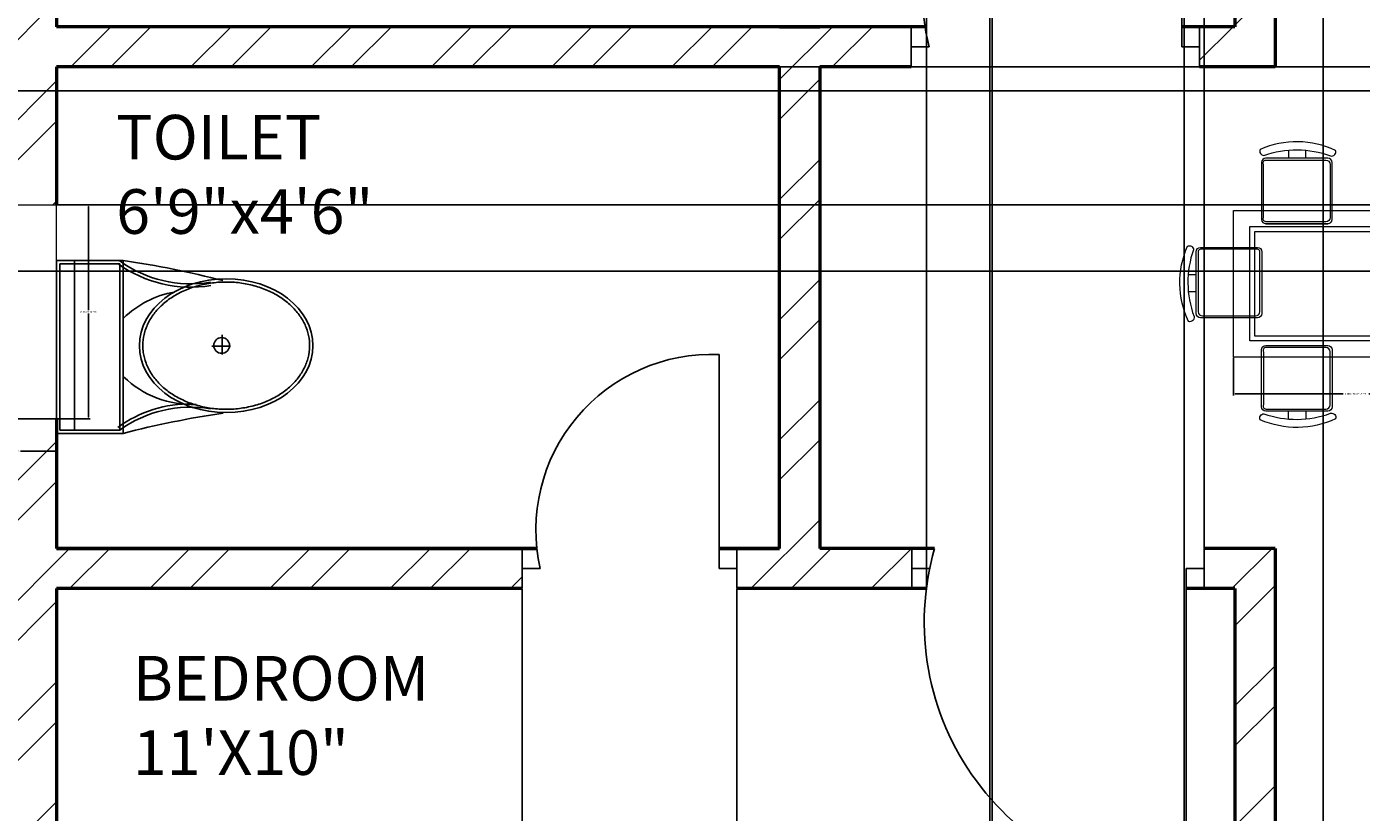
# Model space of a CAD drawing. Units: inches. Extents: x 1980 to 2738, y 1471 to 2568.
# Tile 4 of 22: x 2111 to 2260, y 1790 to 1878. Entities that reach past the tile are written whole.
import ezdxf

# ---------------------------------------------------------------- set-up
doc = ezdxf.new("R2010")
doc.units = ezdxf.units.IN
for name, color, linetype, lineweight in [('A-ANNO-DIMS', 2, 'Continuous', 18), ('A-AREA-IDEN', 7, 'Continuous', 18), ('A-DOOR', 31, 'Continuous', 25), ('A-FLOR-FIXT', 8, 'Continuous', 25), ('A-FURN', 8, 'Continuous', 18), ('A-GLAZ', 141, 'Continuous', 18), ('A-WALL', 7, 'Continuous', 50)]:
    doc.layers.add(name, color=color, linetype=linetype, lineweight=lineweight)
doc.layers.add('A-WALL-PATT', color=9, linetype='Continuous', lineweight=13, true_color=0xd19cc7)
doc.styles.get("Standard").update_dxf_attribs({"font": 'arial.ttf'})
doc.dimstyles.get("Standard").update_dxf_attribs({"dimtxt": 0.18, "dimasz": 0.18, "dimexe": 0.18, "dimexo": 0.0625, "dimgap": 0.09, "dimtad": 0, "dimtih": 1, "dimtoh": 1, "dimdec": 4, "dimzin": 0, "dimdsep": 46, "dimtxsty": 'Standard', "dimcen": 0.09, "dimadec": 0, "dimazin": 0, "dimtfac": 1, "dimtdec": 4, "dimtofl": 0, "dimtmove": 0, "dimatfit": 3, "dimfxl": 1, "dimtolj": 1, "dimtzin": 0, "dimarcsym": 0})

# ---------------------------------------------------------------- blocks, each defined once
blk = doc.blocks.new('A$C31115884')
for p, q in [((257.5, 466.4), (257.5, 523.2)), ((283.1, 497.7), (223.4, 497.7)), ((0, 200), (0, 0)), ((520, 200), (0, 200)), ((10, 190), (10, 10)), ((510, 190), (10, 190)), ((510, 10), (510, 190)), ((520, 0), (520, 200)), ((510, 54.5), (0, 54.5)), ((10, 10), (510, 10)), ((0, 0), (520, 0))]:
    blk.add_line(p, q)
blk.add_circle((255.6, 496.4), 23.6)
for centre, radius, start, end in [((2777.7, -204.6), 2807, 165.4549, 171.7133), ((3237, 905), 2807, 188.2867, 194.5451), ((-294.5, 403.3), 364.7, 324.2091, 9.3499), ((-294.5, 403.3), 374.7, 324.2091, 9.3499), ((805.8, 403.3), 364.7, 170.6501, 215.7909), ((139.5, 406.2), 293.5, 315.8436, 2.6563), ((805.8, 403.3), 374.7, 179.2036, 215.7909), ((383.6, 406.2), 293.5, 190.2774, 224.1564)]:
    blk.add_arc(centre, radius, start, end)
blk.add_ellipse((256.2, 509.9), major_axis=(0, -260.7), ratio=0.772727)
blk.add_open_spline([(256.2, 259.2), (263.1, 259.2), (270, 259.7), (287.8, 262.3), (298.7, 265.1), (319.9, 273.1), (330.2, 278.4), (350.1, 291.1), (359.7, 298.7), (377.7, 315.9), (386.2, 325.5), (401.7, 346.6), (408.8, 358.1), (421.3, 382.5), (426.8, 395.5), (435.9, 422.4), (439.5, 436.4), (444.8, 465.1), (446.5, 479.7), (447.9, 509.2), (447.6, 524), (445, 553.3), (442.7, 567.8), (436.3, 596), (432.1, 609.7), (421.9, 636), (416, 648.6), (402.5, 672.1), (395, 683), (378.6, 703), (369.8, 712.1), (351.1, 728), (341.3, 734.8), (320.9, 746.2), (310.4, 750.7), (288.9, 757.3), (278, 759.4), (256, 761), (245, 760.6), (223.1, 757.2), (212.3, 754.3), (191.1, 746.1), (180.8, 740.7), (160.9, 727.8), (151.4, 720.1), (133.5, 702.7), (125.1, 693), (109.6, 671.7), (102.6, 660.2), (90.2, 635.7), (84.9, 622.7), (76, 595.6), (72.4, 581.6), (67.2, 552.9), (65.6, 538.2), (64.4, 508.8), (64.8, 494), (67.5, 464.7), (69.9, 450.2), (76.6, 422), (80.8, 408.3), (91.1, 382.2), (97.2, 369.7), (110.8, 346.3), (118.4, 335.4), (134.8, 315.6), (143.7, 306.7), (162.4, 290.9), (172.3, 284.2), (192.8, 273), (203.3, 268.6), (224.8, 262.2), (235.8, 260.2), (249.9, 259.3), (253, 259.2), (256.2, 259.2)], degree=3, knots=[0, 0, 0, 0, 0.110105, 0.110105, 0.285049, 0.285049, 0.459994, 0.459994, 0.634938, 0.634938, 0.809882, 0.809882, 0.984827, 0.984827, 1.159771, 1.159771, 1.334715, 1.334715, 1.50966, 1.50966, 1.684604, 1.684604, 1.859549, 1.859549, 2.034493, 2.034493, 2.209437, 2.209437, 2.384382, 2.384382, 2.559326, 2.559326, 2.73427, 2.73427, 2.909215, 2.909215, 3.084159, 3.084159, 3.259103, 3.259103, 3.434048, 3.434048, 3.608992, 3.608992, 3.783936, 3.783936, 3.958881, 3.958881, 4.133825, 4.133825, 4.30877, 4.30877, 4.483714, 4.483714, 4.658658, 4.658658, 4.833603, 4.833603, 5.008547, 5.008547, 5.183491, 5.183491, 5.358436, 5.358436, 5.53338, 5.53338, 5.708324, 5.708324, 5.883269, 5.883269, 6.058213, 6.058213, 6.233158, 6.233158, 6.283185, 6.283185, 6.283185, 6.283185])
blk = doc.blocks.new('TABLE-DINING-RECT')
for points in [[(0, 16.47), (27.45, 16.47), (27.45, 0), (0, 0)], [(0, 16.47), (27.45, 16.47), (27.45, 0), (0, 0)], [(1.83, 14.64), (25.62, 14.64), (25.62, 1.83), (1.83, 1.83)], [(1.83, 14.64), (25.62, 14.64), (25.62, 1.83), (1.83, 1.83)], [(2.38, 14.09), (25.07, 14.09), (25.07, 2.38), (2.38, 2.38)], [(2.38, 14.09), (25.07, 14.09), (25.07, 2.38), (2.38, 2.38)]]:
    blk.add_lwpolyline(points, close=True)
blk = doc.blocks.new('WIN-24IN-WALL')
for p, q in [((4.5, 24), (0, 24)), ((0, 24), (9, 24)), ((0, 24), (0, 0)), ((4.5, 0), (4.5, 24)), ((9, 0), (9, 24)), ((0, 0), (9, 0)), ((9, 0), (4.5, 0))]:
    blk.add_line(p, q)
blk = doc.blocks.new('*D21')
at = {"layer": 'A-ANNO-DIMS', "color": 0, "lineweight": -2, "transparency": 16777216}
for p, q in [((2245.93, 1840.58), (2245.93, 1836.35)), ((2273.38, 1840.58), (2273.38, 1836.35)), ((2246.11, 1836.53), (2258.22, 1836.53)), ((2273.2, 1836.53), (2261.09, 1836.53))]:
    blk.add_line(p, q, dxfattribs=at)
at = {"layer": 'A-ANNO-DIMS', "color": 0, "transparency": 16777216}
for points in [[(2246.11, 1836.56), (2246.11, 1836.5), (2245.93, 1836.53)], [(2273.2, 1836.56), (2273.2, 1836.5), (2273.38, 1836.53)]]:
    blk.add_solid(points, dxfattribs=at)
at = {"layer": 'Defpoints', "color": 0, "transparency": 16777216}
for p in [(2245.93, 1840.64), (2273.38, 1840.64), (2273.38, 1836.53)]:
    blk.add_point(p, dxfattribs=at)
at = {"layer": 'A-ANNO-DIMS', "color": 0, "transparency": 16777216, "insert": (2259.65, 1836.53), "char_height": 0.18, "attachment_point": 5}
blk.add_mtext('\\A1;DINING TABLE 27 TYP.', dxfattribs=at)
blk = doc.blocks.new('*D23')
at = {"layer": 'A-ANNO-DIMS', "color": 0, "lineweight": -2, "transparency": 16777216}
for p, q in [((2114.15, 1857.73), (2117.86, 1857.73)), ((2117.68, 1857.55), (2117.68, 1845.91)), ((2117.68, 1833.91), (2117.68, 1845.54)), ((2114.15, 1833.73), (2117.86, 1833.73))]:
    blk.add_line(p, q, dxfattribs=at)
at = {"layer": 'A-ANNO-DIMS', "color": 0, "transparency": 16777216}
for points in [[(2117.65, 1857.55), (2117.71, 1857.55), (2117.68, 1857.73)], [(2117.65, 1833.91), (2117.71, 1833.91), (2117.68, 1833.73)]]:
    blk.add_solid(points, dxfattribs=at)
at = {"layer": 'Defpoints', "color": 0, "transparency": 16777216}
for p in [(2114.08, 1857.73), (2117.68, 1857.73), (2114.08, 1833.73)]:
    blk.add_point(p, dxfattribs=at)
at = {"layer": 'A-ANNO-DIMS', "color": 0, "transparency": 16777216, "insert": (2117.68, 1845.73), "char_height": 0.18, "attachment_point": 5}
blk.add_mtext('\\A1;WINDOW 24 TYP.', dxfattribs=at)
blk = doc.blocks.new('*D24')
at = {"layer": 'A-ANNO-DIMS', "color": 0, "lineweight": -2, "transparency": 16777216}
for p, q in [((2105.08, 1833.67), (2105.08, 1829.95)), ((2114.08, 1833.67), (2114.08, 1829.95)), ((2105.26, 1830.13), (2109.13, 1830.13)), ((2113.9, 1830.13), (2110.04, 1830.13))]:
    blk.add_line(p, q, dxfattribs=at)
at = {"layer": 'A-ANNO-DIMS', "color": 0, "transparency": 16777216}
for points in [[(2105.26, 1830.16), (2105.26, 1830.1), (2105.08, 1830.13)], [(2113.9, 1830.16), (2113.9, 1830.1), (2114.08, 1830.13)]]:
    blk.add_solid(points, dxfattribs=at)
at = {"layer": 'Defpoints', "color": 0, "transparency": 16777216}
for p in [(2105.08, 1833.73), (2114.08, 1833.73), (2114.08, 1830.13)]:
    blk.add_point(p, dxfattribs=at)
at = {"layer": 'A-ANNO-DIMS', "color": 0, "transparency": 16777216, "insert": (2109.58, 1830.13), "char_height": 0.18, "attachment_point": 5}
blk.add_mtext('\\A1;9 TYP.', dxfattribs=at)
blk = doc.blocks.new('*D40')
at = {"layer": 'A-ANNO-DIMS', "color": 0, "lineweight": -2, "transparency": 16777216}
for p, q in [((2218.65, 2053.14), (2218.65, 1533.71)), ((2298.65, 2053.14), (2298.65, 1533.71)), ((2218.83, 1533.89), (2258.43, 1533.89)), ((2298.47, 1533.89), (2258.87, 1533.89))]:
    blk.add_line(p, q, dxfattribs=at)
at = {"layer": 'A-ANNO-DIMS', "color": 0, "transparency": 16777216}
for points in [[(2218.83, 1533.92), (2218.83, 1533.86), (2218.65, 1533.89)], [(2298.47, 1533.92), (2298.47, 1533.86), (2298.65, 1533.89)]]:
    blk.add_solid(points, dxfattribs=at)
at = {"layer": 'Defpoints', "color": 0, "transparency": 16777216}
for p in [(2218.65, 2053.21), (2298.65, 2053.21), (2298.65, 1533.89)]:
    blk.add_point(p, dxfattribs=at)
at = {"layer": 'A-ANNO-DIMS', "color": 0, "transparency": 16777216, "insert": (2258.65, 1533.89), "char_height": 0.18, "attachment_point": 5}
blk.add_mtext('\\A1;80', dxfattribs=at)
blk = doc.blocks.new('*D44')
at = {"layer": 'A-ANNO-DIMS', "color": 0, "lineweight": -2, "transparency": 16777216}
for p, q in [((2218.88, 1694.77), (2218.88, 2507.54)), ((2219.06, 2507.36), (2229.18, 2507.36)), ((2240.22, 2507.36), (2230.11, 2507.36)), ((2240.4, 1694.77), (2240.4, 2507.54))]:
    blk.add_line(p, q, dxfattribs=at)
at = {"layer": 'A-ANNO-DIMS', "color": 0, "transparency": 16777216}
for points in [[(2219.06, 2507.39), (2219.06, 2507.33), (2218.88, 2507.36)], [(2240.22, 2507.39), (2240.22, 2507.33), (2240.4, 2507.36)]]:
    blk.add_solid(points, dxfattribs=at)
at = {"layer": 'Defpoints', "color": 0, "transparency": 16777216}
for p in [(2240.4, 2507.36), (2218.88, 1694.71), (2240.4, 1694.71)]:
    blk.add_point(p, dxfattribs=at)
at = {"layer": 'A-ANNO-DIMS', "color": 0, "transparency": 16777216, "insert": (2229.64, 2507.36), "char_height": 0.18, "attachment_point": 5}
blk.add_mtext('\\A1;21.525', dxfattribs=at)
blk = doc.blocks.new('*D45')
at = {"layer": 'A-ANNO-DIMS', "color": 0, "lineweight": -2, "transparency": 16777216}
for p, q in [((2255.99, 1694.77), (2255.99, 2507.54)), ((2256.17, 2507.36), (2267.22, 2507.36)), ((2279.21, 2507.36), (2268.15, 2507.36)), ((2279.39, 1694.77), (2279.39, 2507.54))]:
    blk.add_line(p, q, dxfattribs=at)
at = {"layer": 'A-ANNO-DIMS', "color": 0, "transparency": 16777216}
for points in [[(2256.17, 2507.39), (2256.17, 2507.33), (2255.99, 2507.36)], [(2279.21, 2507.39), (2279.21, 2507.33), (2279.39, 2507.36)]]:
    blk.add_solid(points, dxfattribs=at)
at = {"layer": 'Defpoints', "color": 0, "transparency": 16777216}
for p in [(2279.39, 2507.36), (2255.99, 1694.71), (2279.39, 1694.71)]:
    blk.add_point(p, dxfattribs=at)
at = {"layer": 'A-ANNO-DIMS', "color": 0, "transparency": 16777216, "insert": (2267.69, 2507.36), "char_height": 0.18, "attachment_point": 5}
blk.add_mtext('\\A1;23.407', dxfattribs=at)
blk = doc.blocks.new('*D46')
at = {"layer": 'A-ANNO-DIMS', "color": 0, "lineweight": -2, "transparency": 16777216}
for p, q in [((2211.52, 1814.77), (2211.52, 2507.54)), ((2211.7, 2507.36), (2226.69, 2507.36)), ((2242.46, 2507.36), (2227.48, 2507.36)), ((2242.64, 1814.77), (2242.64, 2507.54))]:
    blk.add_line(p, q, dxfattribs=at)
at = {"layer": 'A-ANNO-DIMS', "color": 0, "transparency": 16777216}
for points in [[(2211.7, 2507.39), (2211.7, 2507.33), (2211.52, 2507.36)], [(2242.46, 2507.39), (2242.46, 2507.33), (2242.64, 2507.36)]]:
    blk.add_solid(points, dxfattribs=at)
at = {"layer": 'Defpoints', "color": 0, "transparency": 16777216}
for p in [(2242.64, 2507.36), (2211.52, 1814.71), (2242.64, 1814.71)]:
    blk.add_point(p, dxfattribs=at)
at = {"layer": 'A-ANNO-DIMS', "color": 0, "transparency": 16777216, "insert": (2227.08, 2507.36), "char_height": 0.18, "attachment_point": 5}
blk.add_mtext('\\A1;31.12', dxfattribs=at)
blk = doc.blocks.new('*D47')
at = {"layer": 'A-ANNO-DIMS', "color": 0, "lineweight": -2, "transparency": 16777216}
for p, q in [((2166.25, 1814.64), (2166.25, 1533.71)), ((2190.3, 1814.64), (2190.3, 1533.71)), ((2166.43, 1533.89), (2177.81, 1533.89)), ((2190.12, 1533.89), (2178.74, 1533.89))]:
    blk.add_line(p, q, dxfattribs=at)
at = {"layer": 'A-ANNO-DIMS', "color": 0, "transparency": 16777216}
for points in [[(2166.43, 1533.92), (2166.43, 1533.86), (2166.25, 1533.89)], [(2190.12, 1533.92), (2190.12, 1533.86), (2190.3, 1533.89)]]:
    blk.add_solid(points, dxfattribs=at)
at = {"layer": 'Defpoints', "color": 0, "transparency": 16777216}
for p in [(2166.25, 1814.71), (2190.3, 1814.71), (2190.3, 1533.89)]:
    blk.add_point(p, dxfattribs=at)
at = {"layer": 'A-ANNO-DIMS', "color": 0, "transparency": 16777216, "insert": (2178.28, 1533.89), "char_height": 0.18, "attachment_point": 5}
blk.add_mtext('\\A1;24.044', dxfattribs=at)
blk = doc.blocks.new('*D61')
at = {"layer": 'A-ANNO-DIMS', "color": 0, "lineweight": -2, "transparency": 16777216}
for p, q in [((2114.15, 1873.21), (2689.91, 1873.21)), ((2689.73, 1873.03), (2689.73, 1865.65)), ((2689.73, 1857.91), (2689.73, 1865.29)), ((2114.15, 1857.73), (2689.91, 1857.73))]:
    blk.add_line(p, q, dxfattribs=at)
at = {"layer": 'A-ANNO-DIMS', "color": 0, "transparency": 16777216}
for points in [[(2689.7, 1873.03), (2689.76, 1873.03), (2689.73, 1873.21)], [(2689.7, 1857.91), (2689.76, 1857.91), (2689.73, 1857.73)]]:
    blk.add_solid(points, dxfattribs=at)
at = {"layer": 'Defpoints', "color": 0, "transparency": 16777216}
for p in [(2114.08, 1873.21), (2689.73, 1873.21), (2114.08, 1857.73)]:
    blk.add_point(p, dxfattribs=at)
at = {"layer": 'A-ANNO-DIMS', "color": 0, "transparency": 16777216, "insert": (2689.73, 1865.47), "char_height": 0.18, "attachment_point": 5}
blk.add_mtext('\\A1;15.48', dxfattribs=at)
blk = doc.blocks.new('*D65')
at = {"layer": 'A-ANNO-DIMS', "color": 0, "lineweight": -2, "transparency": 16777216}
for p, q in [((2293.25, 1870.5), (2036.25, 1870.5)), ((2036.43, 1870.32), (2036.43, 1860.58)), ((2036.43, 1850.47), (2036.43, 1860.21)), ((2293.25, 1850.29), (2036.25, 1850.29))]:
    blk.add_line(p, q, dxfattribs=at)
at = {"layer": 'A-ANNO-DIMS', "color": 0, "transparency": 16777216}
for points in [[(2036.4, 1870.32), (2036.46, 1870.32), (2036.43, 1870.5)], [(2036.4, 1850.47), (2036.46, 1850.47), (2036.43, 1850.29)]]:
    blk.add_solid(points, dxfattribs=at)
at = {"layer": 'Defpoints', "color": 0, "transparency": 16777216}
for p in [(2036.43, 1870.5), (2293.31, 1870.5), (2293.31, 1850.29)]:
    blk.add_point(p, dxfattribs=at)
at = {"layer": 'A-ANNO-DIMS', "color": 0, "transparency": 16777216, "insert": (2036.43, 1860.4), "char_height": 0.18, "attachment_point": 5}
blk.add_mtext('\\A1;20.204', dxfattribs=at)

msp = doc.modelspace()

# ---------------------------------------------------------------- hatches: boundary and pattern name
at = {"layer": 'A-WALL-PATT'}
h = msp.add_hatch(dxfattribs=at)
h.set_pattern_fill('ANSI32', color=256)
h.paths.add_polyline_path([(2257.5661, 2416.2064), (2257.5661, 2420.7064), (2250.5833, 2420.7064), (2250.5833, 2462.7064), (2246.0833, 2462.7064), (2246.0833, 2420.7064), (2237.0791, 2420.7064), (2237.0791, 2411.7064), (2246.0833, 2411.7064), (2246.0833, 2291.7064), (2242.6109, 2291.7064), (2242.6109, 2287.2064), (2246.0833, 2287.2064), (2250.5833, 2287.2064), (2250.5833, 2291.7064), (2250.5833, 2411.7064), (2257.5661, 2411.7064)])
h.paths.add_polyline_path([(2387.0396, 2416.2064), (2387.0396, 2420.7064), (2367.5833, 2420.7064), (2367.5833, 2462.7064), (2358.5833, 2462.7064), (2358.5833, 2420.7064), (2329.3087, 2420.7064), (2329.3087, 2411.7064), (2358.5833, 2411.7064), (2358.5833, 2321.7275), (2358.5833, 2309.7064), (2347.3089, 2309.7064), (2293.3089, 2309.7064), (2293.3089, 2259.0771), (2297.8089, 2259.0771), (2297.8089, 2305.2064), (2347.3089, 2305.2064), (2347.3089, 2284.7412), (2351.8089, 2284.7412), (2351.8089, 2305.2064), (2372.3188, 2305.2064), (2372.3761, 2284.3899), (2377.0295, 2284.3899), (2377.0295, 2299.3058), (2377.0295, 2305.2064), (2426.5295, 2305.2064), (2426.5295, 2257.5573), (2431.0295, 2257.5573), (2431.0295, 2309.7064), (2377.0295, 2309.7064), (2367.5833, 2309.7064), (2367.5833, 2321.7275), (2367.5833, 2411.7064), (2387.0396, 2411.7064)])
h.paths.add_polyline_path([(2448.5267, 2416.2064), (2448.5267, 2420.7064), (2423.0396, 2420.7064), (2423.0396, 2411.7064), (2448.5267, 2411.7064)])
h.paths.add_polyline_path([(2130.9128, 2416.2064), (2130.9128, 2420.7064), (2105.0833, 2420.7064), (2105.0833, 2386.6942), (2114.0833, 2386.6942), (2114.0833, 2411.7064), (2130.9128, 2411.7064)])
h.paths.add_polyline_path([(2212.9478, 2420.7064), (2190.9128, 2420.7064), (2190.9128, 2411.7064), (2212.9478, 2411.7064), (2212.9478, 2416.2064)])
h.paths.add_polyline_path([(2114.0833, 2326.6942), (2105.0833, 2326.6942), (2105.0833, 2291.7064), (2081.0833, 2291.7064), (2081.0833, 2287.2064), (2105.0833, 2287.2064), (2105.0833, 2276.1935), (2114.0833, 2276.1935), (2114.0833, 2287.2064), (2166.3825, 2287.2064), (2166.3825, 2289.4564), (2166.3825, 2291.7064), (2114.0833, 2291.7064)])
h.paths.add_polyline_path([(2114.0833, 2252.1935), (2105.0833, 2252.1935), (2105.0833, 2233.2064), (2081.0833, 2233.2064), (2081.0833, 2228.7064), (2105.0833, 2228.7064), (2105.0833, 2213.4478), (2114.0833, 2213.4478), (2114.0833, 2228.7064), (2195.0833, 2228.7064), (2199.5833, 2228.7064), (2208.4455, 2228.7064), (2208.4455, 2230.9564), (2208.4455, 2233.2064), (2199.5833, 2233.2064), (2199.5833, 2287.2064), (2206.8904, 2287.2064), (2206.8904, 2289.4564), (2206.8904, 2291.7064), (2189.446, 2291.7064), (2189.446, 2289.4564), (2189.446, 2287.2064), (2195.0833, 2287.2064), (2195.0833, 2233.2064), (2114.0833, 2233.2064)])
h.paths.add_polyline_path([(2114.0833, 2153.4478), (2109.5833, 2153.4478), (2105.0833, 2153.4478), (2105.0833, 2135.2374), (2114.0833, 2135.2374)], flags=17)
h.paths.add_polyline_path([(2135.9619, 2095.4081), (2140.1805, 2095.4081), (2140.1805, 2104.2064), (2114.0833, 2104.2064), (2114.0833, 2110.3997), (2109.5833, 2110.3997), (2105.0833, 2110.3997), (2105.0833, 2104.2064), (2081.0833, 2104.2064), (2081.0833, 2099.7064), (2105.0833, 2099.7064), (2127.5416, 2099.8532), (2127.5416, 2056.9393), (2136.2133, 2056.9393)], flags=17)
h.paths.add_polyline_path([(2255.4895, 2104.2064), (2250.5833, 2104.2064), (2250.5833, 2233.2064), (2246.0833, 2233.2064), (2242.4941, 2233.2064), (2242.4941, 2228.7064), (2246.0833, 2228.7064), (2246.0833, 2104.2064), (2163.6825, 2104.2064), (2163.6825, 2099.8072), (2163.6825, 2095.4081), (2191.4325, 2095.4081), (2191.4325, 2011.2064), (2186.0833, 2011.2064), (2136.5143, 2010.8824), (2136.3702, 2032.9403), (2131.9559, 2032.9115), (2127.5416, 2032.8826), (2127.5416, 2006.7064), (2105.0833, 2006.7064), (2081.0833, 2006.7064), (2081.0833, 2002.2064), (2105.0833, 2002.2064), (2105.0833, 1995.9329), (2114.0833, 1995.9329), (2114.0833, 2002.2064), (2246.0833, 2002.2064), (2246.0833, 1877.7064), (2242.1358, 1877.7064), (2242.1358, 1873.2064), (2250.5833, 1873.2064), (2250.5833, 2002.2064), (2255.3335, 2002.2064), (2255.3335, 2011.2064), (2195.9325, 2011.2064), (2195.9325, 2095.2064), (2255.4895, 2095.2064), (2255.4895, 2099.5471)])
h.paths.add_polyline_path([(2199.5833, 1873.2064), (2209.827, 1873.2064), (2209.827, 1875.4564), (2209.827, 1877.7064), (2114.0833, 1877.7064), (2114.0833, 1890.0968), (2105.0833, 1890.0968), (2105.0833, 1877.7064), (2081.0833, 1877.7064), (2081.0833, 1873.2064), (2105.0833, 1873.2064), (2105.0833, 1857.7279), (2114.0833, 1857.7279), (2114.0833, 1873.2064), (2195.0833, 1873.2064), (2195.0833, 1819.2064), (2190.298, 1819.2064), (2190.298, 1814.7064), (2209.8976, 1814.7064), (2209.8976, 1816.9564), (2209.8976, 1819.2064), (2199.5833, 1819.2064)])
h.paths.add_polyline_path([(2114.0833, 1814.7064), (2166.2538, 1814.7064), (2166.2538, 1816.9564), (2166.2538, 1819.2064), (2114.0833, 1819.2064), (2114.0833, 1833.7279), (2109.5833, 1833.7279), (2105.0833, 1833.7279), (2105.0833, 1819.2064), (2081.0833, 1819.2064), (2081.0833, 1814.7064), (2105.0833, 1814.7064), (2105.0833, 1782.5516), (2114.0833, 1782.5516)])
h.paths.add_polyline_path([(2114.0833, 1722.5516), (2109.5833, 1722.5516), (2105.0833, 1722.5516), (2105.0833, 1685.7064), (2124.5104, 1685.7064), (2124.5104, 1690.2064), (2124.5104, 1694.7064), (2114.0833, 1694.7064)])
h.paths.add_polyline_path([(2218.8787, 1694.7064), (2184.5104, 1694.7064), (2184.5104, 1685.7064), (2218.8787, 1685.7064), (2218.8787, 1690.2064)])
h.paths.add_polyline_path([(2250.5833, 1819.2064), (2242.6431, 1819.2064), (2242.6431, 1816.9564), (2242.6431, 1814.7064), (2246.0833, 1814.7064), (2246.0833, 1694.7064), (2240.4035, 1694.7064), (2240.4035, 1690.2064), (2240.4035, 1685.7064), (2246.0833, 1685.7064), (2246.0833, 1643.7064), (2250.5833, 1643.7064), (2250.5833, 1685.7064), (2255.9859, 1685.7064), (2255.9859, 1690.2064), (2255.9859, 1694.7064), (2250.5833, 1694.7064)])
h.paths.add_polyline_path([(2297.4764, 1694.7064), (2279.3934, 1694.7064), (2279.3934, 1690.2064), (2279.3934, 1685.7064), (2297.4764, 1685.7064), (2297.4764, 1690.2064)])
h.paths.add_polyline_path([(2377.1596, 1694.7064), (2367.5833, 1694.7064), (2367.5833, 1787.7064), (2431.0295, 1787.7064), (2431.0295, 1792.2064), (2431.0295, 1849.4149), (2428.7795, 1849.4149), (2426.5295, 1849.4149), (2426.5295, 1792.2064), (2421.5833, 1792.2064), (2367.5833, 1792.2064), (2297.8089, 1792.2064), (2297.8089, 1850.2946), (2295.5589, 1850.2946), (2293.3089, 1850.2946), (2293.3089, 1792.2064), (2293.3089, 1787.7064), (2297.8089, 1787.7064), (2358.5833, 1787.7064), (2358.5833, 1694.7064), (2333.4764, 1694.7064), (2333.4764, 1685.7064), (2358.5833, 1685.7064), (2358.5833, 1643.7064), (2367.5833, 1643.7064), (2367.5833, 1685.7064), (2377.1596, 1685.7064)])
h.paths.add_polyline_path([(2442.4912, 1694.7064), (2413.1596, 1694.7064), (2413.1596, 1685.7064), (2442.4912, 1685.7064)])
h.paths.add_polyline_path([(2480.0833, 1814.7064), (2483.4816, 1814.7064), (2483.4816, 1817.9384), (2483.4816, 1819.2064), (2475.5833, 1819.2064), (2475.5833, 1694.7064), (2470.7283, 1694.7064), (2470.7283, 1685.7064), (2475.5833, 1685.7064), (2475.5833, 1643.7064), (2480.0833, 1643.7064), (2480.0833, 1685.7064), (2486.3293, 1685.7064), (2486.3293, 1690.2064), (2486.3293, 1694.7064), (2480.0833, 1694.7064)])
h.paths.add_polyline_path([(2621.0833, 1721.7349), (2612.0833, 1721.7349), (2612.0833, 1694.7064), (2586.1453, 1694.7064), (2586.1453, 1685.7064), (2621.0833, 1685.7064)])
h.paths.add_polyline_path([(2526.1453, 1690.2064), (2526.1453, 1694.7064), (2511.584, 1694.7064), (2511.584, 1690.2064), (2511.584, 1685.7064), (2526.1453, 1685.7064)])
h.paths.add_polyline_path([(2645.0833, 1819.2064), (2621.0833, 1819.2064), (2621.0833, 1835.8527), (2616.5833, 1835.8527), (2612.0833, 1835.8527), (2612.0833, 1819.2064), (2560.2541, 1819.2064), (2560.2541, 1814.7064), (2612.0833, 1814.7064), (2612.0833, 1781.7349), (2621.0833, 1781.7349), (2621.0833, 1814.7064), (2645.0833, 1814.7064)])
h.paths.add_polyline_path([(2645.0833, 1877.7064), (2621.0833, 1877.7064), (2621.0833, 1886.4375), (2612.0833, 1886.4375), (2612.0833, 1877.7064), (2517.1032, 1877.7064), (2517.1032, 1875.4564), (2517.1032, 1873.2064), (2526.5833, 1873.2064), (2526.5833, 1819.2064), (2516.6454, 1819.2064), (2516.6454, 1816.9564), (2516.6454, 1814.7064), (2536.4445, 1814.7064), (2536.4445, 1816.9564), (2536.4445, 1819.2064), (2531.0833, 1819.2064), (2531.0833, 1873.2064), (2612.0833, 1873.2064), (2612.0833, 1859.8527), (2621.0833, 1859.8527), (2621.0833, 1873.2064), (2645.0833, 1873.2064)])
h.paths.add_polyline_path([(2645.0833, 2006.7064), (2621.0833, 2006.7064), (2588.5085, 2006.7064), (2588.5085, 2052.9125), (2579.9045, 2052.9125), (2579.9045, 2011.2064), (2519.9045, 2011.2064), (2519.9045, 2095.2064), (2553.1204, 2095.2064), (2553.1204, 2104.2064), (2480.0833, 2104.2064), (2480.0833, 2228.7064), (2484.3832, 2228.7064), (2484.3832, 2230.9564), (2484.3832, 2233.2064), (2475.5833, 2233.2064), (2475.5833, 2104.2064), (2463.1308, 2104.2064), (2463.1308, 2095.2064), (2501.2463, 2095.2064), (2510.9045, 2095.2064), (2515.4045, 2095.2064), (2515.4045, 2011.2064), (2510.9045, 2011.2064), (2501.2463, 2011.2064), (2462.5957, 2011.2064), (2462.5957, 2002.2064), (2475.5833, 2002.2064), (2475.5833, 1873.2064), (2483.6146, 1873.2064), (2483.6146, 1875.4564), (2483.6146, 1877.7064), (2480.0833, 1877.7064), (2480.0833, 2002.2064), (2612.0833, 2002.2064), (2612.0833, 1996.309), (2621.0833, 1996.309), (2621.0833, 2002.2064), (2645.0833, 2002.2064)])
h.paths.add_polyline_path([(2588.5085, 2099.7277), (2621.0833, 2099.7277), (2645.0833, 2099.7064), (2645.0833, 2104.2064), (2621.0833, 2104.2064), (2621.0833, 2109.0038), (2616.5833, 2109.0038), (2612.0833, 2109.0038), (2612.0833, 2104.2064), (2575.0621, 2104.2064), (2575.0621, 2099.7064), (2575.0621, 2095.2064), (2579.9045, 2095.2064), (2579.9045, 2076.9125), (2588.5085, 2076.9125)], flags=17)
h.paths.add_polyline_path([(2367.5833, 2002.2064), (2373.7228, 2002.2064), (2373.7228, 2006.7064), (2373.7228, 2011.2064), (2350.7889, 2011.2064), (2350.7889, 2006.7064), (2350.7889, 2002.2064), (2358.5833, 2002.2064), (2358.5833, 1877.7064), (2293.3089, 1877.7064), (2293.3089, 1870.4987), (2297.8089, 1870.4987), (2297.8089, 1873.2064), (2347.3089, 1873.2064), (2347.3089, 1847.2208), (2351.8089, 1847.2208), (2351.8089, 1873.2064), (2372.5295, 1873.2064), (2372.5295, 1847.8619), (2377.0295, 1847.8619), (2377.0295, 1873.2064), (2426.5295, 1873.2064), (2426.5295, 1868.7339), (2431.0295, 1868.7339), (2431.0295, 1877.7064), (2367.5833, 1877.7064)])
h.paths.add_polyline_path([(2531.0833, 2287.2064), (2534.2285, 2287.2064), (2534.2285, 2291.7064), (2516.7886, 2291.7064), (2516.7886, 2287.2064), (2526.5833, 2287.2064), (2526.5833, 2233.2064), (2517.9112, 2233.2064), (2517.9112, 2230.9564), (2517.9112, 2228.7064), (2526.5833, 2228.7064), (2531.0833, 2228.7064), (2612.0833, 2228.7064), (2612.0833, 2206.8504), (2621.0833, 2206.8504), (2621.0833, 2228.7064), (2645.0833, 2228.7064), (2645.0833, 2233.2064), (2621.0833, 2233.2064), (2621.0833, 2241.8536), (2616.5833, 2241.8536), (2612.0833, 2241.8536), (2612.0833, 2233.2064), (2531.0833, 2233.2064)])
h.paths.add_polyline_path([(2645.0833, 2291.7064), (2621.0833, 2291.7064), (2621.0833, 2323.0138), (2616.5833, 2323.0138), (2612.0833, 2323.0138), (2612.0833, 2291.7064), (2559.6852, 2291.7064), (2559.6852, 2289.4564), (2559.6852, 2287.2064), (2612.0833, 2287.2064), (2612.0833, 2265.8536), (2621.0833, 2265.8536), (2621.0833, 2287.2064), (2645.0833, 2287.2064)])
h.paths.add_polyline_path([(2621.0833, 2420.7064), (2582.8189, 2420.7064), (2582.8189, 2411.7064), (2612.0833, 2411.7064), (2612.0833, 2383.0138), (2621.0833, 2383.0138)])
h.paths.add_polyline_path([(2480.0833, 2411.7064), (2485.7342, 2411.7064), (2485.7342, 2416.2064), (2485.7342, 2420.7064), (2480.0833, 2420.7064), (2480.0833, 2462.7064), (2475.5833, 2462.7064), (2475.5833, 2420.7064), (2469.4083, 2420.7064), (2469.4083, 2411.7064), (2475.5833, 2411.7064), (2475.5833, 2291.7064), (2475.5833, 2287.2064), (2482.9195, 2287.2064), (2482.9195, 2289.4564), (2482.9195, 2291.7064), (2480.0833, 2291.7064)])
h.paths.add_polyline_path([(2367.5833, 2228.7064), (2431.0295, 2228.7064), (2431.0295, 2233.2064), (2431.0295, 2237.4203), (2428.7795, 2237.4203), (2426.5295, 2237.4203), (2426.5295, 2233.2064), (2377.0295, 2233.2064), (2377.0295, 2260.3837), (2372.4423, 2260.3837), (2372.517, 2233.2635), (2351.8089, 2233.2064), (2351.8089, 2260.7412), (2347.3089, 2260.7412), (2347.3089, 2233.2064), (2297.8089, 2233.2064), (2297.8089, 2236.9324), (2293.3089, 2236.9324), (2293.3089, 2228.7064), (2358.5833, 2228.7064), (2358.5833, 2104.2064), (2353.3665, 2104.2064), (2353.3665, 2095.2064), (2373.8869, 2095.2064), (2373.8869, 2099.7064), (2373.8869, 2104.2064), (2367.5833, 2104.2064)])
h.paths.add_polyline_path([(2321.2323, 2104.2064), (2303.4895, 2104.2064), (2303.4895, 2095.2064), (2321.2323, 2095.2064), (2321.2323, 2099.7064)], flags=0)
h.paths.add_polyline_path([(2415.1308, 2099.7064), (2415.1308, 2104.2064), (2404.81, 2104.2064), (2404.81, 2095.2064), (2415.1308, 2095.2064)], flags=17)
h.paths.add_polyline_path([(2318.6336, 2011.2064), (2303.3335, 2011.2064), (2303.3335, 2002.2064), (2318.6336, 2002.2064)], flags=0)
h.paths.add_polyline_path([(2414.5957, 2011.2064), (2406.2461, 2011.2064), (2406.2461, 2006.7064), (2406.2461, 2002.2064), (2414.5957, 2002.2064)], flags=17)

# ---------------------------------------------------------------- linework, layer by layer
at = {"layer": 'A-DOOR'}
for p, q in [((2240.1358, 1875.4564), (2240.1358, 1911.4564)), ((2209.827, 1877.7064), (2209.827, 1873.2064)), ((2240.8375, 1877.7064), (2240.8375, 1877.7064)), ((2242.1358, 1877.7064), (2242.1358, 1873.2064)), ((2209.827, 1873.2064), (2209.827, 1875.4564)), ((2209.827, 1875.4564), (2211.827, 1875.4564)), ((2242.1358, 1875.4564), (2240.1358, 1875.4564)), ((2242.1358, 1873.2064), (2242.1358, 1875.4564)), ((2188.298, 1816.9564), (2188.298, 1840.9564)), ((2166.2538, 1819.2064), (2166.2538, 1814.7064)), ((2190.298, 1819.2064), (2190.298, 1814.7064)), ((2209.8976, 1819.2064), (2209.8976, 1814.7064)), ((2242.6431, 1814.7064), (2242.6431, 1819.2064)), ((2242.6431, 1819.2064), (2242.6431, 1816.9564)), ((2166.2538, 1814.7064), (2166.2538, 1816.9564)), ((2166.2538, 1816.9564), (2168.2538, 1816.9564)), ((2190.298, 1816.9564), (2188.298, 1816.9564)), ((2190.298, 1814.7064), (2190.298, 1816.9564)), ((2190.298, 1816.9564), (2190.298, 1816.9564)), ((2209.8976, 1814.7064), (2209.8976, 1816.9564)), ((2209.8976, 1816.9564), (2211.8976, 1816.9564)), ((2242.6431, 1816.9564), (2240.6431, 1816.9564)), ((2240.6431, 1816.9564), (2240.6431, 1780.9564))]:
    msp.add_line(p, q, dxfattribs=at)
for centre, radius, start, end in [((2240.1358, 1882.3261), 29.1304, 90, 193.640185), ((2187.4852, 1821.2651), 19.7081, 87.636208, 192.628213), ((2241.2573, 1810.9233), 29.9732, 163.957397, 268.825814)]:
    msp.add_arc(centre, radius, start, end, dxfattribs=at)
at = {"layer": 'A-FURN'}
for points in [[(2249.3251, 1863.2736, -0.17580919), (2256.8005, 1863.217, 0.57839206), (2257.3668, 1863.8397, 0.21452438), (2248.9286, 1863.9529, 0.55201397), (2249.325, 1863.2736, -0.06507904)], [(2249.3251, 1863.2733, -0.17580919), (2256.8005, 1863.2167, 0.57839206), (2257.3668, 1863.8394, 0.21452438), (2248.9286, 1863.9527, 0.55201397), (2249.3251, 1863.2733, -0.06507904)], [(2256.4833, 1862.9736), (2249.5434, 1862.9736, 0.41421356), (2249.0579, 1862.4881), (2249.0579, 1856.1069, 0.41421356), (2249.5434, 1855.6214), (2256.4833, 1855.6214, 0.41421356), (2256.9689, 1856.1069), (2256.9689, 1862.4881, 0.41421356), (2256.4833, 1862.9736)], [(2256.4834, 1862.9733), (2249.5434, 1862.9733, 0.41421356), (2249.0579, 1862.4878), (2249.0579, 1856.1066, 0.41421356), (2249.5434, 1855.6211), (2256.4834, 1855.6211, 0.41421356), (2256.9689, 1856.1066), (2256.9689, 1862.4878, 0.41421356), (2256.4834, 1862.9733)], [(2254.0457, 1862.9736), (2254.0457, 1863.8513, -0.06475861)], [(2254.0457, 1862.9733), (2254.0457, 1863.851, -0.06475861)], [(2241.5043, 1845.2216, -0.57839206), (2240.8816, 1844.6553, -0.21452438), (2240.7684, 1853.0934, -0.55201397), (2241.4477, 1852.697, 0.17580937), (2241.5043, 1845.2216)], [(2241.5043, 1845.2213, -0.57839206), (2240.8816, 1844.655, -0.21452438), (2240.7684, 1853.0931, -0.55201397), (2241.4477, 1852.6967, 0.17580937), (2241.5043, 1845.2213)], [(2241.7477, 1852.4787, -0.41421356), (2242.2333, 1852.9642), (2248.6144, 1852.9642, -0.41421356), (2249.0999, 1852.4787), (2249.0999, 1845.5387, -0.41421356), (2248.6144, 1845.0532), (2242.2333, 1845.0532, -0.41421356), (2241.7477, 1845.5387), (2241.7477, 1852.4787)], [(2241.7477, 1852.4784, -0.41421356), (2242.2333, 1852.9639), (2248.6144, 1852.9639, -0.41421356), (2249.0999, 1852.4784), (2249.0999, 1845.5384, -0.41421356), (2248.6144, 1845.0529), (2242.2333, 1845.0529, -0.41421356), (2241.7477, 1845.5384), (2241.7477, 1852.4784)], [(2241.7477, 1847.9764), (2240.87, 1847.9764, 0.06475861)], [(2241.7477, 1847.9761), (2240.8701, 1847.9761, 0.06475861)], [(2256.4833, 1834.6078), (2249.5434, 1834.6078, -0.41421356), (2249.0579, 1835.0934), (2249.0579, 1841.4745, -0.41421356), (2249.5434, 1841.96), (2256.4833, 1841.96, -0.41421356), (2256.9689, 1841.4745), (2256.9689, 1835.0934, -0.41421356), (2256.4833, 1834.6078)], [(2256.4834, 1834.6076), (2249.5434, 1834.6076, -0.41421356), (2249.0579, 1835.0931), (2249.0579, 1841.4742, -0.41421356), (2249.5434, 1841.9598), (2256.4834, 1841.9598, -0.41421356), (2256.9689, 1841.4742), (2256.9689, 1835.0931, -0.41421356), (2256.4834, 1834.6076)], [(2254.0457, 1834.6078), (2254.0457, 1833.7302, 0.06475861)], [(2254.0457, 1834.6076), (2254.0457, 1833.7299, 0.06475861)], [(2256.8005, 1834.3644, -0.57839206), (2257.3668, 1833.7417, -0.21452438), (2248.9286, 1833.6285, -0.55201397), (2249.325, 1834.3078, 0.17580929), (2256.8005, 1834.3644)], [(2256.8005, 1834.3641, -0.57839206), (2257.3668, 1833.7414, -0.21452438), (2248.9286, 1833.6282, -0.55201397), (2249.3251, 1834.3075, 0.17580929), (2256.8005, 1834.3641)]]:
    msp.add_lwpolyline(points, format="xyb", dxfattribs=at)
for points in [[(2252.1031, 1863.8672), (2252.1031, 1862.9736)], [(2252.1031, 1863.8669), (2252.1031, 1862.9733)], [(2240.8541, 1849.919), (2241.7477, 1849.919)], [(2240.8541, 1849.9187), (2241.7477, 1849.9187)], [(2252.1031, 1833.7142), (2252.1031, 1834.6078)], [(2252.1031, 1833.7139), (2252.1031, 1834.6076)]]:
    msp.add_lwpolyline(points, dxfattribs=at)
for points in [[(2249.5463, 1862.7549), (2256.2646, 1862.7549, -0.41421356), (2256.7501, 1862.2693), (2256.7501, 1856.3257, -0.41421356), (2256.2646, 1855.8401), (2249.5463, 1855.8401, -0.51206948), (2249.2766, 1856.3257), (2249.2766, 1862.2693, -0.51206948)], [(2249.5464, 1862.7546), (2256.2646, 1862.7546, -0.41421356), (2256.7501, 1862.269), (2256.7501, 1856.3254, -0.41421356), (2256.2646, 1855.8398), (2249.5464, 1855.8398, -0.51206948), (2249.2766, 1856.3254), (2249.2766, 1862.269, -0.51206948)], [(2241.9665, 1852.4757), (2241.9665, 1845.7575, 0.41421356), (2242.452, 1845.2719), (2248.3957, 1845.2719, 0.41421356), (2248.8812, 1845.7575), (2248.8812, 1852.4757, 0.51206948), (2248.3957, 1852.7455), (2242.452, 1852.7455, 0.51206948)], [(2241.9665, 1852.4754), (2241.9665, 1845.7572, 0.41421356), (2242.452, 1845.2716), (2248.3957, 1845.2716, 0.41421356), (2248.8812, 1845.7572), (2248.8812, 1852.4754, 0.51206948), (2248.3957, 1852.7452), (2242.452, 1852.7452, 0.51206948)], [(2249.5463, 1834.8266), (2256.2646, 1834.8266, 0.41421356), (2256.7501, 1835.3121), (2256.7501, 1841.2558, 0.41421356), (2256.2646, 1841.7413), (2249.5463, 1841.7413, 0.51206948), (2249.2766, 1841.2558), (2249.2766, 1835.3121, 0.51206948)], [(2249.5464, 1834.8263), (2256.2646, 1834.8263, 0.41421356), (2256.7501, 1835.3118), (2256.7501, 1841.2555, 0.41421356), (2256.2646, 1841.741), (2249.5464, 1841.741, 0.51206948), (2249.2766, 1841.2555), (2249.2766, 1835.3118, 0.51206948)]]:
    msp.add_lwpolyline(points, format="xyb", close=True, dxfattribs=at)
at = {"layer": 'A-WALL'}
for p, q in [((2246.0833, 2002.2064), (2246.0833, 1877.7064)), ((2250.5833, 2002.2064), (2250.5833, 1873.2064)), ((2114.0833, 1902.4872), (2114.0833, 1877.7064)), ((2211.374, 1877.7064), (2114.0833, 1877.7064)), ((2195.0833, 1877.7064), (2199.5833, 1877.7064)), ((2246.0833, 1877.7064), (2240.1358, 1877.7064)), ((2114.0833, 1873.2064), (2114.0833, 1857.7279)), ((2195.0833, 1873.2064), (2114.0833, 1873.2064)), ((2195.0833, 1819.2064), (2195.0833, 1873.2064)), ((2199.5833, 1873.2064), (2199.5833, 1819.2064)), ((2209.827, 1873.2064), (2199.5833, 1873.2064)), ((2250.5833, 1873.2064), (2242.1358, 1873.2064)), ((2114.0833, 1833.7279), (2114.0833, 1819.2064)), ((2114.0833, 1819.2064), (2167.8849, 1819.2064)), ((2167.8849, 1819.2064), (2114.0833, 1819.2064)), ((2195.0833, 1819.2064), (2188.298, 1819.2064)), ((2188.298, 1819.2064), (2195.0833, 1819.2064)), ((2212.4514, 1819.2064), (2199.5833, 1819.2064)), ((2250.5833, 1819.2064), (2242.6431, 1819.2064)), ((2250.5833, 1819.2064), (2250.5833, 1694.7064)), ((2114.0833, 1814.7064), (2114.0833, 1782.5516)), ((2166.2538, 1814.7064), (2114.0833, 1814.7064)), ((2211.5238, 1814.7064), (2190.298, 1814.7064)), ((2246.0833, 1814.7064), (2240.6431, 1814.7064)), ((2246.0833, 1814.7064), (2246.0833, 1694.7064))]:
    msp.add_line(p, q, dxfattribs=at)

# ---------------------------------------------------------------- block references
at = {"layer": 'A-FLOR-FIXT', "xscale": 0.0372717239612423, "yscale": 0.0372717239612423, "zscale": 0.0372717239612423, "rotation": 270}
msp.add_blockref('A$C31115884', (2114.0833, 1851.4926), dxfattribs=at)
at = {"layer": 'A-FURN'}
msp.add_blockref('TABLE-DINING-RECT', (2245.9301, 1840.645), dxfattribs=at)
at = {"layer": 'A-GLAZ'}
msp.add_blockref('WIN-24IN-WALL', (2105.083, 1833.7283), dxfattribs=at)

# ---------------------------------------------------------------- texts
at = {"layer": 'A-AREA-IDEN', "char_height": 5, "attachment_point": 1}
for s, width, insert in [('TOILET\\P6\'9"x4\'6"', 69.580447, (2120.7725, 1867.817)), ('BEDROOM\\P11\'X10"', 100.531108, (2122.6461, 1807.156))]:
    msp.add_mtext_dynamic_manual_height_columns(s, width=width, gutter_width=12.5, heights=[0], dxfattribs=dict(at, insert=insert))

# ---------------------------------------------------------------- dimensions: what is measured, and where the dimension line sits
at = {"layer": 'A-ANNO-DIMS'}
for base, p1, p2, override, picture, middle in [((2242.6431, 2507.3564), (2211.5238, 1814.7064), (2242.6431, 1814.7064), {"dimdec": 2, "dimlfac": 1, "dimrnd": 0, "dimzin": 0, "dimdsep": 46, "dimlunit": 2}, '*D46', (2227.0835, 2507.3564)), ((2240.4035, 2507.3564), (2218.8787, 1694.7064), (2240.4035, 1694.7064), {"dimdec": 3, "dimlfac": 1, "dimrnd": 0, "dimzin": 0, "dimdsep": 46, "dimlunit": 2}, '*D44', (2229.6411, 2507.3564)), ((2279.39337, 2507.35642), (2255.98588, 1694.70642), (2279.39337, 1694.70642), {"dimdec": 3, "dimlfac": 1, "dimrnd": 0, "dimzin": 0, "dimdsep": 46, "dimlunit": 2}, '*D45', (2267.68962, 2507.35642)), ((2298.6516, 1533.8857), (2218.6516, 2053.2064), (2298.6516, 2053.2064), {"dimdec": 0, "dimlfac": 1, "dimrnd": 0, "dimzin": 0, "dimdsep": 46, "dimlunit": 2}, '*D40', (2258.6516, 1533.8857)), ((2190.298, 1533.8857), (2166.2538, 1814.7064), (2190.298, 1814.7064), {"dimdec": 3, "dimlfac": 1, "dimrnd": 0, "dimzin": 0, "dimdsep": 46, "dimlunit": 2}, '*D47', (2178.2759, 1533.8857))]:
    dim = msp.add_linear_dim(base=base, p1=p1, p2=p2, dimstyle='Standard', override=override, dxfattribs=at)
    dim.commit()
    dim.dimension.update_dxf_attribs({"geometry": picture, "text_midpoint": middle})
for base, p1, p2, override, picture, middle in [((2689.7333, 1873.2064), (2114.0833, 1857.7279), (2114.0833, 1873.2064), {"dimdec": 2, "dimlfac": 1, "dimrnd": 0, "dimzin": 0, "dimdsep": 46, "dimlunit": 2}, '*D61', (2689.7333, 1865.4672)), ((2036.4333, 1870.4987), (2293.3089, 1850.2946), (2293.3089, 1870.4987), {"dimdec": 3, "dimlfac": 1, "dimrnd": 0, "dimzin": 0, "dimdsep": 46, "dimlunit": 2}, '*D65', (2036.4333, 1860.3966))]:
    dim = msp.add_linear_dim(base=base, p1=p1, p2=p2, angle=90, dimstyle='Standard', override=override, dxfattribs=at)
    dim.commit()
    dim.dimension.update_dxf_attribs({"geometry": picture, "text_midpoint": middle})
dim = msp.add_linear_dim(base=(2117.6833, 1857.7279), p1=(2114.0833, 1833.7279), p2=(2114.0833, 1857.7279), angle=90, text='WINDOW <> TYP.', dimstyle='Standard', override={"dimdec": 0, "dimlfac": 1, "dimrnd": 0, "dimzin": 0, "dimdsep": 46, "dimlunit": 2}, dxfattribs=at)
dim.commit()
dim.dimension.update_dxf_attribs({"geometry": '*D23', "text_midpoint": (2117.6833, 1845.7279)})
for base, p1, p2, text, picture, middle in [((2273.376, 1836.528), (2245.9303, 1840.6449), (2273.376, 1840.6449), 'DINING TABLE <> TYP.', '*D21', (2259.6532, 1836.528)), ((2114.0833, 1830.1279), (2105.0833, 1833.7279), (2114.0833, 1833.7279), '<> TYP.', '*D24', (2109.5833, 1830.1279))]:
    dim = msp.add_linear_dim(base=base, p1=p1, p2=p2, text=text, dimstyle='Standard', override={"dimdec": 0, "dimlfac": 1, "dimrnd": 0, "dimzin": 0, "dimdsep": 46, "dimlunit": 2}, dxfattribs=at)
    dim.commit()
    dim.dimension.update_dxf_attribs({"geometry": picture, "text_midpoint": middle})

doc.saveas('drawing.dxf')
